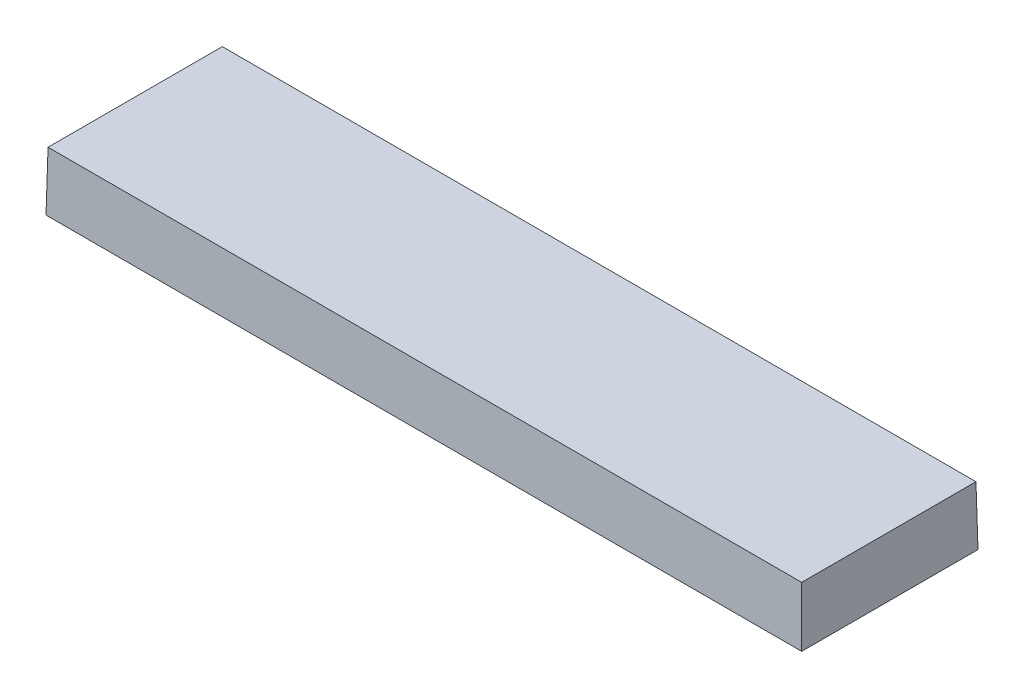
SolidWorks part; units mm, degrees
material "Plain Carbon Steel"
ref_plane "Front Plane" through (0, 0, 0) normal (0, 0, 1) x (1, 0, 0)
ref_plane "Top Plane" through (0, 0, 0) normal (0, 1, 0) x (1, 0, 0)
ref_plane "Right Plane" through (0, 0, 0) normal (1, 0, 0) x (0, 0, -1)
sketch "Cotter Profile 90x25" plane through (0, 0, 0) normal (0, 1, 0) x (1, 0, 0)
  line L1 (-45, 10.5) -> (45, 10.5)
  line L2 (-45, 10.5) -> (-45, -10.5)
  line L3 (-45, -10.5) -> (45, -10.5)
  line L4 (45, 10.5) -> (45, -10.5)
  line L5 (-45, 10.5) -> (45, -10.5) construction
  line L6 (-45, -10.5) -> (45, 10.5) construction
  point P0 (0, 0)
  dimension "D1" = 21
  dimension "D2" = 90
extrude "Cotter Body 7mm Drafted 1°" add sketch "Cotter Profile 90x25" along normal blind 7 draft 1
